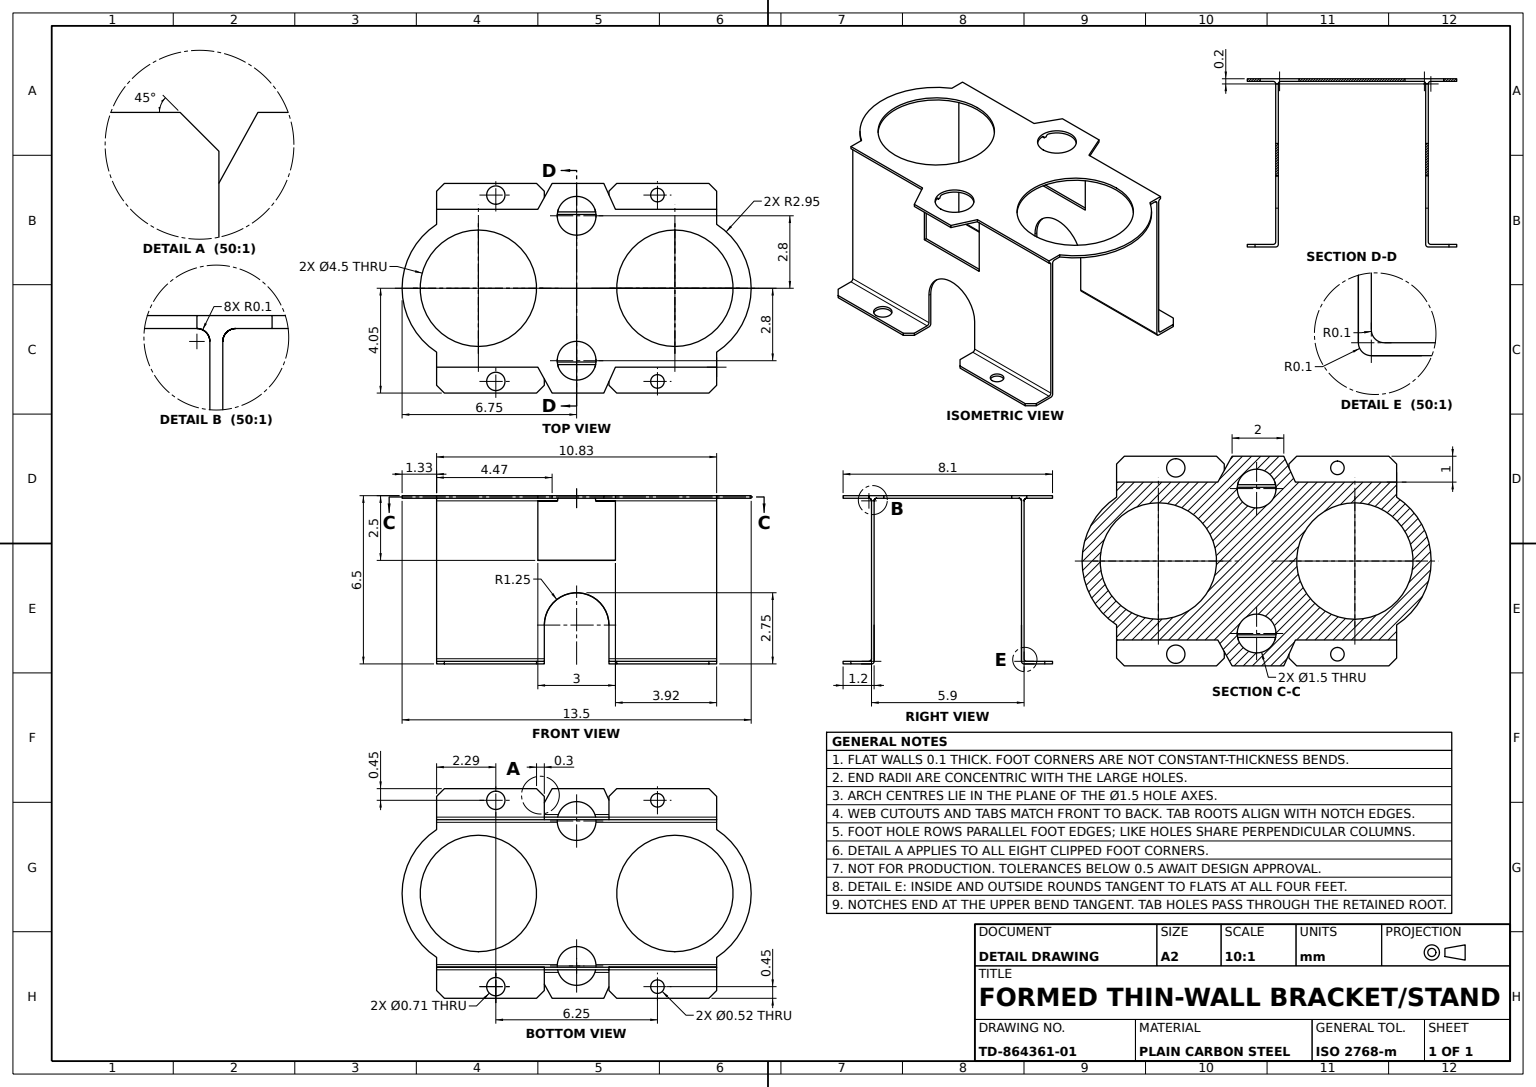
SolidWorks part; units mm, degrees
material "Plain Carbon Steel"
ref_plane "Front Plane" through (0, 0, 0) normal (0, 0, 1) x (1, 0, 0)
ref_plane "Top Plane" through (0, 0, 0) normal (0, 1, 0) x (1, 0, 0)
ref_plane "Right Plane" through (0, 0, 0) normal (1, 0, 0) x (0, 0, -1)
sketch "Channel Profile Sketch" plane through (0, 0, 0) normal (0, 0, 1) x (1, 0, 0)
  line L0 (-4.05, 0) -> (4.05, 0) construction
  line L1 (-2.85, 0.1) -> (-2.85, 6.3)
  line L2 (-2.75, 6.4) -> (2.75, 6.4)
  line L3 (2.85, 6.3) -> (2.85, 0.1)
  line L4 (2.95, 0) -> (4.05, 0)
  line L5 (4.05, 0) -> (4.05, 0.1)
  line L6 (4.05, 0.1) -> (3.05, 0.1)
  line L7 (2.95, 0.2) -> (2.95, 6.3)
  line L8 (3.05, 6.4) -> (4.05, 6.4)
  line L9 (4.05, 6.4) -> (4.05, 6.5)
  line L10 (4.05, 6.5) -> (-4.05, 6.5)
  line L11 (-4.05, 6.5) -> (-4.05, 6.4)
  line L12 (-4.05, 6.4) -> (-3.05, 6.4)
  line L13 (-2.95, 6.3) -> (-2.95, 0.2)
  line L14 (-3.05, 0.1) -> (-4.05, 0.1)
  line L15 (-4.05, 0.1) -> (-4.05, 0)
  line L16 (-4.05, 0) -> (-2.95, 0)
  arc A0 (-2.95, 0.2) -> (-3.05, 0.1) centre (-3.05, 0.2) cw
  arc A1 (3.05, 0.1) -> (2.95, 0.2) centre (3.05, 0.2) cw
  arc A2 (2.95, 0) -> (2.85, 0.1) centre (2.95, 0.1) cw
  arc A3 (2.85, 6.3) -> (2.75, 6.4) centre (2.75, 6.3) ccw
  arc A4 (-2.75, 6.4) -> (-2.85, 6.3) centre (-2.75, 6.3) ccw
  arc A5 (-2.85, 0.1) -> (-2.95, 0) centre (-2.95, 0.1) cw
  arc A6 (-2.95, 6.3) -> (-3.05, 6.4) centre (-3.05, 6.3) ccw
  arc A7 (2.95, 6.3) -> (3.05, 6.4) centre (3.05, 6.3) cw
  point P4 (0, 0)
  point P14 (-3.5, 0)
  point P27 (2.85, 0)
  point P34 (-2.85, 0)
  dimension "D14" = 0.1
  dimension "D15" = 0.1
  dimension "D1" = 8.1
  dimension "D2" = 2.85
  dimension "D3" = 2.85
  dimension "D4" = 4.05
  dimension "D5" = 0.1
  dimension "D6" = 0.1
  dimension "D7" = 0.1
  dimension "D8" = 0.1
  dimension "D9" = 0.1
  dimension "D10" = 0.1
  dimension "D11" = 0.1
  dimension "D12" = 4.05
  dimension "D13" = 4.05
  dimension "D16" = 6.5
  dimension "D17" = 6.5
extrude "Bracket Channel Body" add sketch "Channel Profile Sketch" along normal mid plane 10.83
sketch "Side Arch Cut A Sketch" plane through (2.95, 0, 0) normal (1, 0, 0) x (0, 0, -1)
  line L0 (-1.25, 1.5) -> (-1.25, 0)
  line L1 (-5.415, 0) -> (5.415, 0) construction
  line L2 (0, 0) -> (0, 6.4) construction
  line L3 (-5.415, 6.4) -> (5.415, 6.4) construction
  line L4 (-1.25, 0) -> (1.25, 0)
  line L5 (1.25, 0) -> (1.25, 1.5)
  arc A0 (1.25, 1.5) -> (-1.25, 1.5) centre (0, 1.5) ccw
  point P1 (0, 2.75)
  dimension "D1" = 2.5
  dimension "D2" = 2.75
extrude "Side Arch Cut A" cut sketch "Side Arch Cut A Sketch" against normal blind 10.83
sketch "Side Window Cut Sketch" plane through (-2.95, 0, 0) normal (-1, 0, 0) x (0, 0, 1)
  line L0 (-1.25, 0.2) -> (-1.25, 0)
  line L1 (-1.25, 0) -> (1.25, 0)
  line L2 (1.25, 0) -> (1.25, 0.2)
  line L3 (-1.25, 0.2) -> (1.25, 0.2) construction
  line L4 (1.25, 0.2) -> (-1.25, 0.2)
extrude "Side Window Cut" cut sketch "Side Window Cut Sketch" against normal blind 10.83
sketch "Side Arch Cut B Sketch" plane through (2.95, 0, 0) normal (1, 0, 0) x (0, 0, -1)
  line L0 (-5.415, 6.3) -> (5.415, 6.3) construction
  line L1 (-1.5, 6.3) -> (1.5, 6.3)
  line L2 (-1.5, 6.3) -> (-1.5, 4)
  line L3 (-1.5, 4) -> (1.5, 4)
  line L4 (1.5, 6.3) -> (1.5, 4)
  line L5 (-1.5, 6.3) -> (1.5, 4) construction
  line L6 (-1.5, 4) -> (1.5, 6.3) construction
  line L7 (-5.415, 6.5) -> (5.415, 6.5) construction
  point P4 (0, 5.15)
  dimension "D1" = 2.5
  dimension "D2" = 3
extrude "Side Arch Cut B" cut sketch "Side Arch Cut B Sketch" against normal blind 10.83
sketch "Top Plate Lugs Sketch" plane through (0, 6.5, 0) normal (0, 1, 0) x (1, 0, 0)
  line L0 (0, 6.75) -> (0, 5.415) construction
  line L1 (-2.4687, 5.415) -> (-1.5666, 5.415)
  line L4 (-2.95, 3.6945) -> (-2.9481, 3.6945) construction
  line L5 (-2.4687, -5.415) -> (-1.5666, -5.415)
  line L7 (2.9481, 3.6945) -> (2.95, 3.6945) construction
  line L8 (1.5666, -5.415) -> (2.4687, -5.415)
  line L9 (0, 3.6945) -> (0, -5.415) construction
  line L10 (0, -6.05) -> (0, -6.75) construction
  line L11 (1.5666, 5.415) -> (2.4687, 5.415)
  line L12 (-4.05, -5.415) -> (-4.05, 5.415) construction
  arc A1 (2.4687, 5.415) -> (-2.4687, 5.415) centre (0, 3.8) ccw
  arc A2 (-2.4687, -5.415) -> (2.4687, -5.415) centre (0, -3.8) ccw
  arc A3 (-1.5666, -5.415) -> (1.5666, -5.415) centre (0, -3.8) ccw
  arc A4 (1.5666, 5.415) -> (-1.5666, 5.415) centre (0, 3.8) ccw
  point P15 (-1.125, -3.8)
  dimension "D1" = 1.5813
  dimension "D2" = 5.9
  dimension "D3" = 4.5
  dimension "D4" = 5.9
  dimension "D5" = 2.4834
  dimension "D6" = 6.75
  dimension "D7" = 6.75
  dimension "D8" = 2.925
  dimension "D9" = 9.1095
  dimension "D10" = 9.215
extrude "Top Plate Lugs" add sketch "Top Plate Lugs Sketch" against normal blind 0.1
sketch "Lug Trim Cut Sketch" plane through (0, 6.5, 0) normal (0, 1, 0) x (1, 0, 0)
  circle A0 centre (0, 3.8) radius 2.25
  circle A1 centre (0, -3.8) radius 2.25
  dimension "D1" = 4.5
extrude "Lug Trim Cut" cut sketch "Lug Trim Cut Sketch" against normal blind 0.1
sketch "Large Holes 2xD2.8 Sketch" plane through (0, 6.5, 0) normal (0, 1, 0) x (1, 0, 0)
  line L0 (-4.05, 0) -> (4.05, 0) construction
  line L1 (4.05, -5.415) -> (4.05, 5.415) construction
  circle A0 centre (2.8, 0) radius 0.75
  circle A1 centre (-2.8, 0) radius 0.75
  point P6 (0, 0)
  dimension "D3" = 1.5
  dimension "D4" = 1.5
  dimension "D1" = 2.8
  dimension "D2" = 2.8
extrude "Large Holes 2xD2.8" cut sketch "Large Holes 2xD2.8 Sketch" against normal blind 0.1
sketch "Hole Cut A Sketch" plane through (0, 6.4, 0) normal (0, 1, 0) x (1, 0, 0)
  circle A0 centre (2.8, 0) radius 0.75
  dimension "D1" = 1.5
extrude "Hole Cut A" cut sketch "Hole Cut A Sketch" against normal blind 0.1
sketch "Profile Trim Cut Sketch" plane through (0, 6.5, 0) normal (0, 1, 0) x (1, 0, 0)
  line L1 (-4.05, 1.0516) -> (-3.05, 1.5)
  line L2 (-3.05, 1.5) -> (-3.05, 5.415)
  line L4 (-4.05, -0.9484) -> (-3.05, -1.5)
  line L9 (-2.4687, 5.415) -> (-4.05, 5.415) construction
  line L10 (-3.05, 5.415) -> (-4.05, 5.415)
  line L11 (-4.05, 5.415) -> (-4.05, 1.0516)
  line L13 (-2.4687, -5.415) -> (-4.05, -5.415) construction
  line L14 (-3.05, -5.415) -> (-4.05, -5.415)
  line L15 (4.05, -5.415) -> (4.05, 5.415) construction
  line L16 (-4.05, -0.9484) -> (-4.05, -5.415)
  line L17 (-3.05, -1.5) -> (-3.05, -5.415)
  line L18 (0, 7.331) -> (0, -7.0684) construction
  line L19 (3.05, -1.5) -> (3.05, -5.415)
  line L20 (4.05, -0.9484) -> (4.05, -5.415)
  line L21 (4.05, -5.415) -> (2.4687, -5.415) construction
  line L22 (3.05, -5.415) -> (4.05, -5.415)
  line L24 (4.05, 5.415) -> (4.05, 1.0516)
  line L25 (3.05, 5.415) -> (4.05, 5.415)
  line L26 (4.05, -0.9484) -> (3.05, -1.5)
  line L27 (3.05, 1.5) -> (3.05, 5.415)
  line L28 (4.05, 1.0516) -> (3.05, 1.5)
  dimension "D1" = 2
  dimension "D2" = 3
  dimension "D3" = 1
  dimension "D4" = 4.4666
extrude "Profile Trim Cut" cut sketch "Profile Trim Cut Sketch" against normal blind 0.1
sketch "Small Holes 2xD0.45 Sketch" plane through (0, 0.1, 0) normal (0, 1, 0) x (1, 0, 0)
  line L0 (4.05, 1.25) -> (4.05, 5.415) construction
  line L1 (4.05, -5.415) -> (4.05, -1.25) construction
  line L2 (0, 8.9298) -> (0, -9.2344) construction
  circle A0 centre (3.6, 3.125) radius 0.2615
  circle A1 centre (3.6, -3.125) radius 0.3546
  circle A2 centre (-3.6, -3.125) radius 0.3546
  circle A3 centre (-3.6, 3.125) radius 0.2615
  dimension "D5" = 0.7091
  dimension "D6" = 0.5231
  dimension "D1" = 0.45
  dimension "D2" = 0.45
  dimension "D3" = 3.125
  dimension "D4" = 3.125
extrude "Small Holes 2xD0.45" cut sketch "Small Holes 2xD0.45 Sketch" against normal blind 0.1
sketch "Hole Cut B Sketch" plane through (0, 6.4, 0) normal (0, 1, 0) x (1, 0, 0)
  circle A0 centre (-2.8, 0) radius 0.75
  dimension "D1" = 1.5
extrude "Hole Cut B" cut sketch "Hole Cut B Sketch" against normal blind 0.1
chamfer "Edge Chamfer 0.3" distance 0.3 angle 45 1 edges at (4.05, 0.05, 5.415)
chamfer "Arch Edge Chamfer 0.3" distance 0.3 angle 45 7 edges at (-4.05, 0.05, 5.415) (-4.05, 0.05, 1.25) (-4.05, 0.05, -1.25) (-4.05, 0.05, -5.415) (4.05, 0.05, -5.415) (4.05, 0.05, -1.25) (4.05, 0.05, 1.25)
